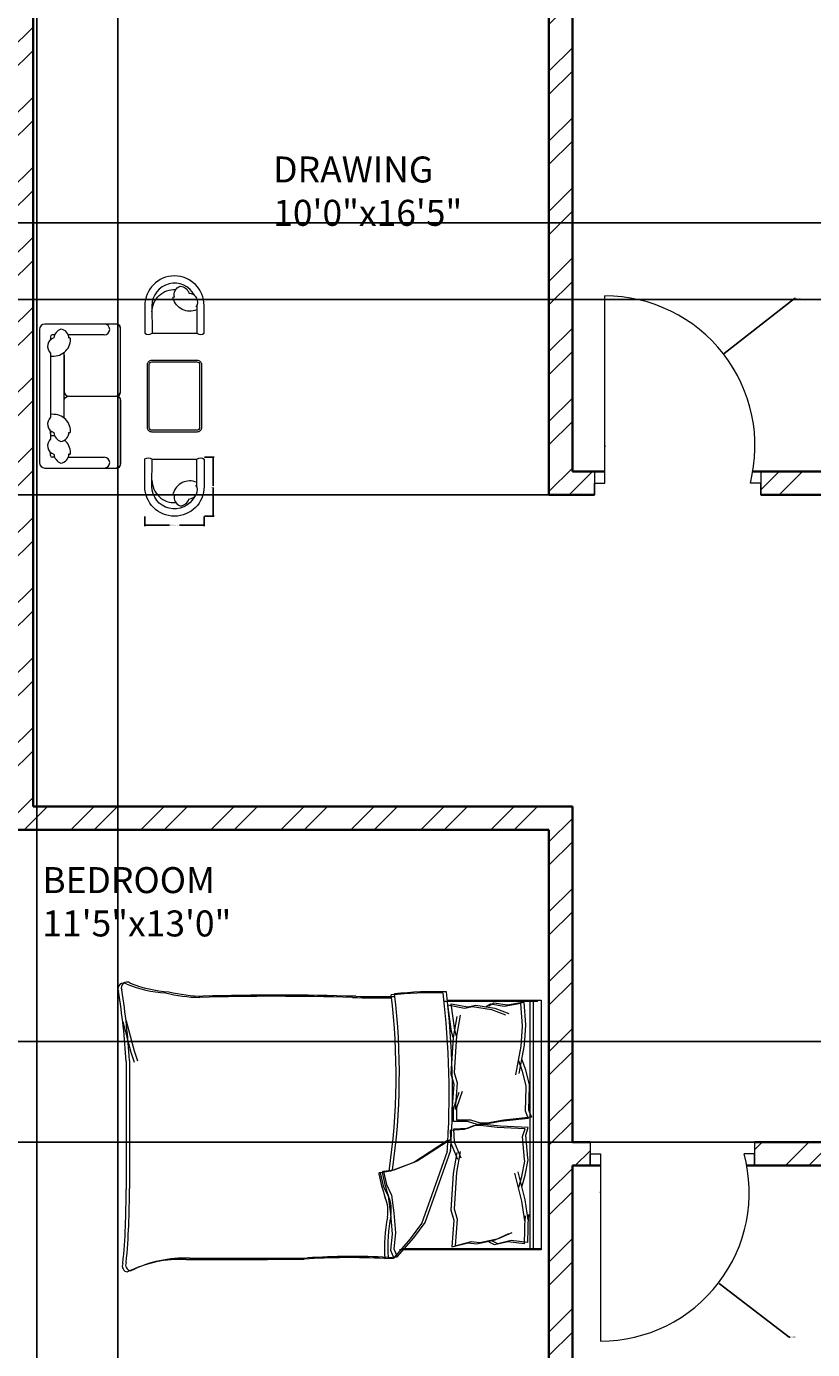
# Model space of a CAD drawing. Units: inches. Extents: x 2008 to 2657, y 1077 to 2165.
# Tile 6 of 16: x 2306 to 2457, y 1312 to 1567. Entities that reach past the tile are written whole.
import ezdxf

# ---------------------------------------------------------------- set-up
doc = ezdxf.new("R2010")
doc.units = ezdxf.units.IN
for name, color, linetype, lineweight in [('A-ANNO-DIMS', 2, 'Continuous', 18), ('A-AREA-IDEN', 4, 'Continuous', 18), ('A-DOOR', 11, 'Continuous', 18), ('A-FURN', 8, 'Continuous', 13), ('A-WALL', 7, 'Continuous', 35)]:
    doc.layers.add(name, color=color, linetype=linetype, lineweight=lineweight)
doc.layers.add('A-WALL-PATT', color=30, linetype='Continuous', lineweight=13, true_color=0xf8991e)
doc.styles.get("Standard").update_dxf_attribs({"font": 'arial.ttf'})
doc.dimstyles.get("Standard").update_dxf_attribs({"dimtxt": 0.18, "dimasz": 0.18, "dimexe": 0.18, "dimexo": 0.0625, "dimgap": 0.09, "dimtad": 0, "dimtih": 1, "dimtoh": 1, "dimdec": 4, "dimzin": 0, "dimdsep": 46, "dimtxsty": 'Standard', "dimcen": 0.09, "dimadec": 0, "dimazin": 0, "dimtfac": 1, "dimtdec": 4, "dimtofl": 0, "dimtmove": 0, "dimatfit": 3, "dimfxl": 1, "dimtolj": 1, "dimtzin": 0, "dimarcsym": 0})

# ---------------------------------------------------------------- blocks, each defined once
blk = doc.blocks.new('A$C1352')
at = {"color": 0}
for points in [[(0.003, 0.053), (0.003, 0.553, -0.414214), (0.053, 0.603), (0.753, 0.603, -0.414214), (0.803, 0.553), (0.803, 0.053, -0.414214), (0.753, 0.003), (0.053, 0.003, -0.414214)], [(0.023, 0.053), (0.023, 0.553, -0.414214), (0.053, 0.583), (0.753, 0.583, -0.414214), (0.783, 0.553), (0.783, 0.053, -0.414214), (0.753, 0.023), (0.053, 0.023, -0.414214)]]:
    blk.add_lwpolyline(points, format="xyb", close=True, dxfattribs=at)
blk = doc.blocks.new('BED-DOUBLE')
for p, q in [((0, 51.49), (0.64, 51.49)), ((0, 3.48), (0, 51.49)), ((0, 51.27), (26.61, 51.27)), ((0, 51.27), (26.61, 51.27)), ((0.64, 51.49), (27.25, 51.49)), ((0.64, 51.49), (27.25, 51.49)), ((1.53, 3.48), (1.53, 51.27)), ((1.53, 3.48), (1.53, 51.27)), ((2.17, 3.7), (2.17, 51.49)), ((2.17, 3.7), (2.17, 51.49)), ((17.21, 50.93), (14.07, 50.15)), ((17.21, 50.93), (14.07, 50.15)), ((16.81, 45.8), (17.21, 50.93)), ((16.81, 45.8), (17.21, 50.93)), ((27.75, 52.87), (24.5, 49.16)), ((27.75, 52.87), (24.5, 49.16)), ((28.39, 53.1), (25.14, 49.39)), ((28.39, 53.1), (25.14, 49.39)), ((29.49, 52.95), (27.75, 52.87, 3.87)), ((29.49, 52.95), (27.75, 52.87, 3.87)), ((28.37, 51.33), (27.75, 52.87)), ((28.37, 51.33), (27.75, 52.87)), ((28.06, 48.23), (28.37, 51.33)), ((28.06, 48.23), (28.37, 51.33)), ((30.13, 53.18), (28.39, 53.1, 3.87)), ((30.13, 53.18), (28.39, 53.1, 3.87)), ((29, 51.56), (28.39, 53.1)), ((29, 51.56), (28.39, 53.1)), ((28.7, 48.46), (29, 51.56)), ((28.7, 48.46), (29, 51.56)), ((2.56, 50.11), (2.46, 44.71)), ((2.56, 50.11), (2.46, 44.71)), ((2.56, 50.11), (5.77, 49.73)), ((2.56, 50.11), (5.77, 49.73)), ((3.2, 50.34), (3.1, 44.94)), ((3.2, 50.34), (3.1, 44.94)), ((3.2, 50.34), (6.41, 49.96)), ((3.2, 50.34), (6.41, 49.96)), ((8.26, 49.31), (5.58, 48.13)), ((8.26, 49.31), (5.58, 48.13)), ((5.77, 49.73), (8.34, 50.33)), ((5.77, 49.73), (8.34, 50.33)), ((8.9, 49.54), (6.22, 48.36)), ((8.9, 49.54), (6.22, 48.36)), ((6.41, 49.96), (8.98, 50.56)), ((6.41, 49.96), (8.98, 50.56)), ((11.83, 50.11), (8.26, 49.31)), ((11.83, 50.11), (8.26, 49.31)), ((8.34, 50.33), (9.38, 49.82)), ((8.34, 50.33), (9.38, 49.81)), ((12.47, 50.34), (8.9, 49.54)), ((12.47, 50.34), (8.9, 49.54)), ((8.98, 50.56), (10.02, 50.04)), ((8.98, 50.56), (10.02, 50.04)), ((13.43, 49.92), (11.83, 50.11)), ((13.43, 49.92), (11.83, 50.11)), ((14.07, 50.15), (12.47, 50.34)), ((14.07, 50.15), (12.47, 50.34)), ((16.57, 50.7), (13.43, 49.92)), ((16.57, 50.7), (13.43, 49.92)), ((16.17, 45.57), (16.57, 50.7)), ((16.17, 45.57), (16.57, 50.7)), ((24.5, 49.16), (22.33, 46.22)), ((24.5, 49.16), (22.33, 46.22)), ((25.14, 49.39), (22.97, 46.45)), ((25.14, 49.39), (22.97, 46.45)), ((29, 44.59), (28.7, 48.46)), ((29, 44.59), (28.7, 48.46)), ((3.1, 44.94), (3.18, 45.94)), ((3.1, 44.94), (3.18, 45.94)), ((3.18, 45.94), (3.71, 42.14)), ((3.18, 45.94), (3.71, 42.14)), ((22.33, 46.22), (20.32, 40.64)), ((22.33, 46.22), (20.32, 40.64)), ((22.97, 46.45), (20.96, 40.87)), ((22.97, 46.45), (20.96, 40.87)), ((28.37, 44.36), (28.06, 48.23)), ((28.37, 44.36), (28.06, 48.23)), ((2.46, 44.71), (2.54, 45.71)), ((2.46, 44.71), (2.54, 45.71)), ((2.54, 45.71), (3.07, 41.91)), ((2.54, 45.71), (3.07, 41.91)), ((16.73, 43.61), (16.17, 45.57)), ((16.73, 43.61), (16.17, 45.57)), ((16.3, 36.6), (16.73, 43.61)), ((16.3, 36.6), (16.73, 43.61)), ((17.37, 43.84), (16.81, 45.8)), ((17.37, 43.83), (16.81, 45.8)), ((16.93, 36.83), (17.37, 43.84)), ((16.93, 36.82), (17.37, 43.83)), ((28.83, 40.95), (28.37, 44.36)), ((28.83, 40.95), (28.37, 44.36)), ((29.47, 41.18), (29, 44.59)), ((29.47, 41.18), (29, 44.59)), ((3.07, 41.91), (4.42, 36.5)), ((3.07, 41.91), (4.42, 36.5)), ((3.71, 42.14), (5.06, 36.72)), ((3.71, 42.14), (5.06, 36.72)), ((20.96, 40.87), (18.02, 32.54)), ((20.96, 40.87), (18.02, 32.53)), ((29.76, 38.94), (28.83, 40.95)), ((29.76, 38.94), (28.83, 40.95)), ((30.4, 39.17), (29.47, 41.18)), ((30.4, 39.17), (29.47, 41.18)), ((3.67, 39.2), (3.08, 37.14)), ((3.67, 39.2), (3.08, 37.14)), ((4.31, 39.43), (3.72, 37.36)), ((4.31, 39.43), (3.72, 37.36)), ((20.32, 40.64), (17.38, 32.31)), ((20.32, 40.64), (17.38, 32.31)), ((30.38, 36.46), (29.76, 38.94)), ((30.38, 36.46), (29.76, 38.94)), ((31.02, 36.69), (30.4, 39.17)), ((31.02, 36.69), (30.4, 39.17)), ((79.25, 15.06), (79.25, 39.68)), ((79.25, 15.06), (79.25, 39.68)), ((79.88, 15.29), (79.88, 39.91)), ((79.88, 15.29), (79.88, 39.91)), ((3.08, 37.14), (2.54, 34.21)), ((3.08, 37.14), (2.54, 34.2)), ((3.72, 37.36), (3.18, 34.43)), ((3.72, 37.36), (3.18, 34.43)), ((15.63, 32.56), (16.3, 36.6)), ((15.63, 32.56), (16.3, 36.6)), ((16.27, 32.79), (16.93, 36.83)), ((16.27, 32.79), (16.93, 36.82)), ((23.88, 34.45), (28.37, 36.15)), ((23.88, 34.45), (28.37, 36.15)), ((24.52, 34.68), (29, 36.38)), ((24.52, 34.68), (29, 36.38)), ((28.37, 36.15), (30.38, 36.46)), ((28.37, 36.15), (30.38, 36.46)), ((29, 36.38), (31.02, 36.69)), ((29, 36.38), (31.02, 36.69)), ((2.54, 34.21), (2.56, 33.88)), ((2.54, 34.2), (2.56, 33.88)), ((2.56, 33.88), (2.98, 29.46)), ((2.56, 33.88), (2.98, 29.46)), ((3.18, 34.43), (3.2, 34.11)), ((3.18, 34.43), (3.2, 34.11)), ((3.2, 34.11), (3.62, 29.68)), ((3.2, 34.11), (3.62, 29.68)), ((16.74, 30.75), (15.45, 33.82)), ((16.74, 30.75), (15.45, 33.82)), ((17.38, 30.98), (16.09, 34.05)), ((17.38, 30.98), (16.09, 34.05)), ((17.38, 30.26), (23.88, 34.45)), ((17.38, 30.26), (23.88, 34.45)), ((18.02, 30.49), (24.52, 34.68)), ((18.02, 30.49), (24.52, 34.68)), ((16.89, 28.3), (16.74, 30.75)), ((16.89, 28.3), (16.74, 30.75)), ((17.53, 28.53), (17.38, 30.98)), ((17.53, 28.53), (17.38, 30.98)), ((2.98, 29.46), (2.49, 27.98)), ((2.98, 29.46), (2.49, 27.98)), ((3.62, 29.68), (3.13, 28.21)), ((3.62, 29.68), (3.13, 28.21)), ((3.13, 28.21), (8.51, 27.96)), ((3.13, 28.21), (8.51, 27.96)), ((12.38, 27.44), (14.22, 28.13)), ((12.38, 27.44), (14.22, 28.13)), ((13.02, 27.66), (14.86, 28.36)), ((13.02, 27.66), (14.86, 28.36)), ((14.22, 28.13), (16.89, 28.3)), ((14.22, 28.13), (16.89, 28.3)), ((14.86, 28.36), (17.53, 28.53)), ((14.86, 28.36), (17.53, 28.53)), ((1.87, 25.98), (7.22, 26.56)), ((1.87, 25.98), (7.22, 26.56)), ((2.45, 24.54), (1.87, 25.98)), ((2.45, 24.54), (1.87, 25.98)), ((2.49, 27.98), (7.87, 27.73)), ((2.49, 27.98), (7.87, 27.73)), ((2.51, 26.21), (7.86, 26.79)), ((2.51, 26.21), (7.86, 26.79)), ((3.09, 24.77), (2.51, 26.21)), ((3.09, 24.77), (2.51, 26.21)), ((7.22, 26.56), (10.4, 27.14)), ((7.22, 26.56), (10.4, 27.14)), ((7.86, 26.79), (11.04, 27.37)), ((7.86, 26.79), (11.04, 27.37)), ((7.87, 27.73), (11.08, 27.36)), ((7.87, 27.73), (11.08, 27.36)), ((8.51, 27.96), (11.72, 27.58)), ((8.51, 27.96), (11.72, 27.58)), ((10.4, 27.14), (11.7, 27.14)), ((10.4, 27.14), (11.7, 27.14)), ((11.04, 27.37), (12.34, 27.37)), ((11.04, 27.37), (12.34, 27.37)), ((11.08, 27.36), (12.38, 27.44)), ((11.08, 27.36), (12.38, 27.44)), ((11.7, 27.14), (13.58, 26.56)), ((11.7, 27.14), (13.58, 26.56)), ((11.72, 27.58), (13.02, 27.66)), ((11.72, 27.58), (13.02, 27.66)), ((12.34, 27.37), (14.22, 26.79)), ((12.34, 27.37), (14.22, 26.79)), ((13.58, 26.56), (16.26, 26.56)), ((13.58, 26.56), (16.26, 26.56)), ((14.22, 26.79), (16.9, 26.79)), ((14.22, 26.79), (16.9, 26.79)), ((16.26, 26.56), (16.26, 24.1)), ((16.26, 26.56), (16.26, 24.1)), ((16.9, 26.79), (16.9, 24.33)), ((16.9, 26.79), (16.9, 24.33)), ((2.3, 20.09), (2.45, 24.54)), ((2.3, 20.09), (2.45, 24.54)), ((2.94, 20.32), (3.09, 24.77)), ((2.94, 20.32), (3.09, 24.77)), ((16.26, 24.1), (15.17, 20.96)), ((16.26, 24.1), (15.17, 20.96)), ((16.9, 24.33), (15.81, 21.19)), ((16.9, 24.33), (15.81, 21.19)), ((16.17, 19.38), (16.57, 24.52)), ((16.17, 19.38), (16.57, 24.52)), ((16.81, 19.61), (17.21, 24.74)), ((16.81, 19.61), (17.21, 24.74)), ((2.3, 19.77), (2.3, 20.09)), ((2.3, 19.77), (2.3, 20.09)), ((3.03, 16.88), (2.3, 19.77)), ((3.03, 16.88), (2.3, 19.77)), ((2.94, 20), (2.94, 20.32)), ((2.94, 20), (2.94, 20.32)), ((3.67, 17.11), (2.94, 20)), ((3.67, 17.11), (2.94, 20)), ((3.96, 12.34), (4.97, 17.83)), ((3.96, 12.34), (4.97, 17.83)), ((16.73, 17.42), (16.17, 19.38)), ((16.73, 17.42), (16.17, 19.38)), ((17.37, 17.65), (16.81, 19.61)), ((17.37, 17.65), (16.81, 19.61)), ((3.75, 14.86), (3.03, 16.88)), ((3.75, 14.86), (3.03, 16.88)), ((3.32, 12.11), (4.33, 17.6)), ((3.32, 12.11), (4.33, 17.6)), ((4.39, 15.08), (3.67, 17.11)), ((4.39, 15.08), (3.67, 17.11)), ((16.3, 10.41), (16.73, 17.42)), ((16.3, 10.41), (16.73, 17.42)), ((16.93, 10.64), (17.37, 17.65)), ((16.93, 10.64), (17.37, 17.65)), ((3.03, 8.29), (3.32, 12.11)), ((3.03, 8.29), (3.32, 12.11)), ((3.67, 8.51), (3.96, 12.34)), ((3.67, 8.51), (3.96, 12.34)), ((15.63, 6.38), (16.3, 10.41)), ((15.63, 6.38), (16.3, 10.41)), ((16.27, 6.61), (16.93, 10.64)), ((16.27, 6.61), (16.93, 10.64)), ((16.3, 10.41), (16.62, 9.28)), ((16.3, 10.41), (16.62, 9.28)), ((16.93, 10.64), (17.26, 9.51)), ((16.93, 10.64), (17.26, 9.51)), ((3.01, 8.18), (3.03, 8.29)), ((3.01, 8.18), (3.03, 8.29)), ((3.34, 3.9), (3.01, 8.18)), ((3.34, 3.9), (3.01, 8.18)), ((3.65, 8.41), (3.67, 8.51)), ((3.65, 8.41), (3.67, 8.51)), ((3.98, 4.13), (3.65, 8.41)), ((3.98, 4.13), (3.65, 8.41)), ((16.62, 9.28), (17.34, 4.18)), ((16.62, 9.28), (17.34, 4.18)), ((17.26, 9.51), (17.98, 4.41)), ((17.26, 9.51), (17.98, 4.41)), ((8.96, 5.05), (6.21, 6.06)), ((8.96, 5.05), (6.21, 6.06)), ((9.59, 5.28), (6.85, 6.29)), ((9.59, 5.28), (6.85, 6.29)), ((13.21, 4.7), (9.59, 5.28)), ((13.21, 4.7), (9.59, 5.28)), ((18.11, 3.48), (0, 3.48)), ((18.11, 3.48), (0, 3.48)), ((18.75, 3.7), (0.64, 3.7)), ((18.75, 3.7), (0.64, 3.7)), ((3.32, 3.9), (6.5, 4.47)), ((3.32, 3.89), (6.5, 4.47)), ((3.96, 4.12), (7.14, 4.7)), ((3.96, 4.12), (7.14, 4.7)), ((6.5, 4.47), (9.1, 4.04)), ((6.5, 4.47), (9.1, 4.04)), ((7.14, 4.7), (9.74, 4.27)), ((7.14, 4.7), (9.74, 4.27)), ((12.57, 4.47), (8.96, 5.05)), ((12.57, 4.47), (8.96, 5.05)), ((9.1, 4.04), (10.11, 4.62)), ((9.1, 4.04), (10.11, 4.62)), ((9.74, 4.27), (10.75, 4.85)), ((9.74, 4.27), (10.75, 4.85)), ((14.16, 4.76), (12.57, 4.47)), ((14.16, 4.76), (12.57, 4.47)), ((14.8, 4.99), (13.21, 4.7)), ((14.8, 4.99), (13.21, 4.7)), ((17.34, 4.18), (14.16, 4.76)), ((17.34, 4.18), (14.16, 4.76)), ((17.98, 4.41), (14.8, 4.99)), ((17.98, 4.41), (14.8, 4.99))]:
    blk.add_line(p, q)
for centre, radius, start, end in [((68.67, 76.16), 23.07, 267.4714, 296.4681), ((68.67, 76.16), 23.07, 267.4714, 296.4681), ((69.31, 76.39), 23.07, 267.4714, 296.4681), ((69.31, 76.39), 23.07, 267.4714, 296.4681), ((78.87, 54.41), 1.1, 332.6588, 86.02), ((78.87, 54.41), 1.1, 332.6588, 86.02), ((212.28, 41.15), 133.04, 174.4998, 180.6351), ((212.28, 41.15), 133.04, 174.4998, 180.6351), ((79.51, 54.64), 1.1, 332.6588, 86.02), ((79.51, 54.64), 1.1, 332.6588, 86.02), ((212.92, 41.38), 133.04, 174.4998, 180.6351), ((212.92, 41.38), 133.04, 174.4998, 180.6351), ((-6.66, 51.33), 36.18, 349.8763, 2.5657), ((-6.66, 51.33), 36.18, 349.8763, 2.5657), ((36.32, 182.27), 129.5, 266.9791, 273.8365), ((36.32, 182.27), 129.5, 266.9791, 273.8365), ((-6.02, 51.56), 36.18, 349.8763, 2.5657), ((-6.02, 51.56), 36.18, 349.8763, 2.5657), ((36.95, 182.49), 129.5, 266.9791, 273.8365), ((36.95, 182.49), 129.5, 266.9791, 273.8365), ((67.82, -4508.74), 4561.86, 90.00217, 90.28689), ((67.82, -4508.74), 4561.86, 90.00217, 90.28689), ((68.46, -4508.51), 4561.86, 90.00217, 90.28689), ((68.46, -4508.51), 4561.86, 90.00217, 90.28689), ((35.07, 43.74), 6.22, 168.6608, 203.7384), ((35.07, 43.74), 6.22, 168.6608, 203.7384), ((35.71, 43.97), 6.22, 168.6608, 203.7384), ((35.71, 43.97), 6.22, 168.6608, 203.7384), ((1.48, 31.15), 29.65, 10.6617, 19.8806), ((1.48, 31.15), 29.65, 10.6617, 19.8806), ((2.12, 31.38), 29.65, 10.6617, 19.8806), ((2.12, 31.38), 29.65, 10.6617, 19.8806), ((156.32, 17.76), 129.02, 171.7845, 186.9006), ((156.32, 17.76), 129.02, 171.7845, 186.9006), ((156.96, 17.98), 129.02, 171.7845, 186.9006), ((156.96, 17.98), 129.02, 171.7845, 186.9006), ((30.44, 36.64), 0.185, 250.2464, 1.1377), ((30.44, 36.64), 0.185, 250.2464, 1.1377), ((31.08, 36.87), 0.185, 250.2464, 1.1377), ((31.08, 36.86), 0.185, 250.2464, 1.1377), ((182.05, 21.36), 164.97, 176.0865, 186.7821), ((182.05, 21.36), 164.97, 176.0865, 186.7821), ((182.69, 21.59), 164.97, 176.0865, 186.7821), ((182.69, 21.59), 164.97, 176.0865, 186.7821), ((-23.07, -16.99), 106.46, 13.3832, 17.7053), ((-23.07, -16.99), 106.46, 13.3832, 17.7053), ((201.48, 21.66), 121.76, 182.9958, 189.4091), ((201.48, 21.66), 121.76, 182.9958, 189.4091), ((-23.71, -17.22), 106.46, 13.3832, 17.7053), ((-23.71, -17.22), 106.46, 13.3832, 17.7053), ((200.84, 21.43), 121.76, 182.9958, 189.4091), ((200.84, 21.43), 121.76, 182.9958, 189.4091), ((31.17, -167.31), 170.11, 88.4762, 91.0082), ((31.17, -167.31), 170.11, 88.4762, 91.0082), ((31.81, -167.08), 170.11, 88.4762, 91.0082), ((31.81, -167.08), 170.11, 88.4762, 91.0082), ((50.61, 484.82), 482.31, 268.2277, 271.7185), ((50.61, 484.82), 482.31, 268.2277, 271.7185), ((51.25, 485.05), 482.31, 268.2277, 271.7185), ((51.25, 485.05), 482.31, 268.2277, 271.7185), ((64.52, -26.9), 29.63, 76.0648, 88.9113), ((64.52, -26.9), 29.63, 76.0648, 88.9113), ((65.15, -26.67), 29.63, 76.0648, 88.9113), ((65.15, -26.67), 29.63, 76.0648, 88.9113), ((20.1, 85.16), 83.31, 268.7218, 275.604), ((20.1, 85.16), 83.31, 268.7218, 275.604), ((20.74, 85.39), 83.31, 268.7218, 275.604), ((20.74, 85.39), 83.31, 268.7218, 275.604), ((70.28, -21.66), 23.56, 67.9751, 86.652), ((70.28, -21.66), 23.56, 67.9751, 86.652), ((70.92, -21.43), 23.56, 67.9751, 86.652), ((70.92, -21.43), 23.56, 67.9751, 86.652), ((79.72, 1.09), 1.09, 236.1736, 23.4781), ((79.72, 1.09), 1.09, 236.1736, 23.4781), ((80.36, 1.32), 1.09, 236.1736, 23.4781), ((80.36, 1.32), 1.09, 236.1736, 23.4781)]:
    blk.add_arc(centre, radius, start, end)
blk = doc.blocks.new('LOUNGE-CHAIR')
blk.add_line((1.39, 5.54), (1.38, 0.26))
at = {"ltscale": 0.03}
blk.add_lwpolyline([(1.38, 0.26, -0.369229), (0, 0.27), (0, 5.54, -1), (11.42, 5.53), (11.42, 0.25, -0.369229), (10.03, 0.26)], format="xyb", close=True, dxfattribs=at)
blk.add_lwpolyline([(1.88, 7.54, -0.785087), (10.04, 5.53), (10.03, 0.26)], format="xyb")
for centre, radius, start, end in [((3.01, 6.23), 1.73, 92.9922, 214.1401), ((4.77, 7.34), 1.95, 94.9999, 161.3534), ((3.98, 7.61), 1.78, 346.6403, 69.4695), ((5.71, 4.32), 4.33, 359.9461, 93.658), ((5.71, 5.54), 4.33, 178.8536, 179.9461), ((2.75, 7.82), 3.35, 247.0143, 344.2857), ((5.79, 7.01), 0.207, 330.6238, 113.7423)]:
    blk.add_arc(centre, radius, start, end)
blk = doc.blocks.new('*D15')
at = {"layer": 'A-ANNO-DIMS', "color": 0, "lineweight": -2, "transparency": 16777216}
for p, q in [((2329, 1472.5), (2329, 1470.67)), ((2329.18, 1470.85), (2333.76, 1470.85)), ((2340.24, 1470.85), (2335.66, 1470.85)), ((2340.42, 1472.5), (2340.42, 1470.67))]:
    blk.add_line(p, q, dxfattribs=at)
at = {"layer": 'A-ANNO-DIMS', "color": 0, "transparency": 16777216}
for points in [[(2329.18, 1470.88), (2329.18, 1470.82), (2329, 1470.85)], [(2340.24, 1470.88), (2340.24, 1470.82), (2340.42, 1470.85)]]:
    blk.add_solid(points, dxfattribs=at)
at = {"layer": 'Defpoints', "color": 0, "transparency": 16777216}
for p in [(2329, 1472.56), (2329, 1470.85), (2340.42, 1472.56)]:
    blk.add_point(p, dxfattribs=at)
at = {"layer": 'A-ANNO-DIMS', "color": 0, "transparency": 16777216, "insert": (2334.71, 1470.85), "char_height": 0.18, "attachment_point": 5}
blk.add_mtext('\\A1;CHAIR 11 TYP.', dxfattribs=at)
blk = doc.blocks.new('*D16')
at = {"layer": 'A-ANNO-DIMS', "color": 0, "lineweight": -2, "transparency": 16777216}
for p, q in [((2340.49, 1483.9), (2342.32, 1483.9)), ((2342.14, 1483.72), (2342.14, 1478.41)), ((2342.14, 1472.74), (2342.14, 1478.05)), ((2340.49, 1472.56), (2342.32, 1472.56))]:
    blk.add_line(p, q, dxfattribs=at)
at = {"layer": 'A-ANNO-DIMS', "color": 0, "transparency": 16777216}
for points in [[(2342.11, 1483.72), (2342.17, 1483.72), (2342.14, 1483.9)], [(2342.11, 1472.74), (2342.17, 1472.74), (2342.14, 1472.56)]]:
    blk.add_solid(points, dxfattribs=at)
at = {"layer": 'Defpoints', "color": 0, "transparency": 16777216}
for p in [(2340.42, 1483.9), (2340.42, 1472.56), (2342.14, 1472.56)]:
    blk.add_point(p, dxfattribs=at)
at = {"layer": 'A-ANNO-DIMS', "color": 0, "transparency": 16777216, "insert": (2342.14, 1478.23), "char_height": 0.18, "attachment_point": 5}
blk.add_mtext('\\A1;11 TYP.', dxfattribs=at)
blk = doc.blocks.new('*D31')
at = {"layer": 'A-ANNO-DIMS', "color": 0, "lineweight": -2, "transparency": 16777216}
for p, q in [((2076.26, 1562.18), (2076.26, 1140.44)), ((2576.76, 1188.61), (2576.76, 1140.44)), ((2076.44, 1140.62), (2326.12, 1140.62)), ((2576.58, 1140.62), (2326.91, 1140.62))]:
    blk.add_line(p, q, dxfattribs=at)
at = {"layer": 'A-ANNO-DIMS', "color": 0, "transparency": 16777216}
for points in [[(2076.44, 1140.65), (2076.44, 1140.59), (2076.26, 1140.62)], [(2576.58, 1140.65), (2576.58, 1140.59), (2576.76, 1140.62)]]:
    blk.add_solid(points, dxfattribs=at)
at = {"layer": 'Defpoints', "color": 0, "transparency": 16777216}
for p in [(2076.26, 1562.24), (2576.76, 1188.67), (2576.76, 1140.62)]:
    blk.add_point(p, dxfattribs=at)
at = {"layer": 'A-ANNO-DIMS', "color": 0, "transparency": 16777216, "insert": (2326.51, 1140.62), "char_height": 0.18, "attachment_point": 5}
blk.add_mtext('\\A1;500.5', dxfattribs=at)
blk = doc.blocks.new('*D53')
at = {"layer": 'A-ANNO-DIMS', "color": 0, "lineweight": -2, "transparency": 16777216}
for p, q in [((2406.7, 1613.17), (2028.03, 1613.17)), ((2028.21, 1612.99), (2028.21, 1545.11)), ((2028.21, 1476.85), (2028.21, 1544.74)), ((2406.7, 1476.67), (2028.03, 1476.67))]:
    blk.add_line(p, q, dxfattribs=at)
at = {"layer": 'A-ANNO-DIMS', "color": 0, "transparency": 16777216}
for points in [[(2028.18, 1612.99), (2028.24, 1612.99), (2028.21, 1613.17)], [(2028.18, 1476.85), (2028.24, 1476.85), (2028.21, 1476.67)]]:
    blk.add_solid(points, dxfattribs=at)
at = {"layer": 'Defpoints', "color": 0, "transparency": 16777216}
for p in [(2406.76, 1613.17), (2028.21, 1476.67), (2406.76, 1476.67)]:
    blk.add_point(p, dxfattribs=at)
at = {"layer": 'A-ANNO-DIMS', "color": 0, "transparency": 16777216, "insert": (2028.21, 1544.92), "char_height": 0.18, "attachment_point": 5}
blk.add_mtext('\\A1;136.5', dxfattribs=at)
blk = doc.blocks.new('*D64')
at = {"layer": 'A-ANNO-DIMS', "color": 0, "lineweight": -2, "transparency": 16777216}
for p, q in [((2308.25, 1777.08), (2308.25, 1140.44)), ((2323.83, 1776.91), (2323.83, 1140.44)), ((2308.43, 1140.62), (2315.59, 1140.62)), ((2323.65, 1140.62), (2316.49, 1140.62))]:
    blk.add_line(p, q, dxfattribs=at)
at = {"layer": 'A-ANNO-DIMS', "color": 0, "transparency": 16777216}
for points in [[(2308.43, 1140.65), (2308.43, 1140.59), (2308.25, 1140.62)], [(2323.65, 1140.65), (2323.65, 1140.59), (2323.83, 1140.62)]]:
    blk.add_solid(points, dxfattribs=at)
at = {"layer": 'Defpoints', "color": 0, "transparency": 16777216}
for p in [(2308.25, 1777.15), (2323.83, 1776.97), (2323.83, 1140.62)]:
    blk.add_point(p, dxfattribs=at)
at = {"layer": 'A-ANNO-DIMS', "color": 0, "transparency": 16777216, "insert": (2316.04, 1140.62), "char_height": 0.18, "attachment_point": 5}
blk.add_mtext('\\A1;15.572', dxfattribs=at)
blk = doc.blocks.new('*D68')
at = {"layer": 'A-ANNO-DIMS', "color": 0, "lineweight": -2, "transparency": 16777216}
for p, q in [((2572.2, 1371.57), (2028.03, 1371.57)), ((2028.21, 1371.39), (2028.21, 1362.05)), ((2028.21, 1352.35), (2028.21, 1361.69)), ((2572.2, 1352.17), (2028.03, 1352.17))]:
    blk.add_line(p, q, dxfattribs=at)
at = {"layer": 'A-ANNO-DIMS', "color": 0, "transparency": 16777216}
for points in [[(2028.18, 1371.39), (2028.24, 1371.39), (2028.21, 1371.57)], [(2028.18, 1352.35), (2028.24, 1352.35), (2028.21, 1352.17)]]:
    blk.add_solid(points, dxfattribs=at)
at = {"layer": 'Defpoints', "color": 0, "transparency": 16777216}
for p in [(2028.21, 1371.57), (2572.26, 1371.57), (2572.26, 1352.17)]:
    blk.add_point(p, dxfattribs=at)
at = {"layer": 'A-ANNO-DIMS', "color": 0, "transparency": 16777216, "insert": (2028.21, 1361.87), "char_height": 0.18, "attachment_point": 5}
blk.add_mtext('\\A1;19.394', dxfattribs=at)
blk = doc.blocks.new('*D69')
at = {"layer": 'A-ANNO-DIMS', "color": 0, "lineweight": -2, "transparency": 16777216}
for p, q in [((2109.32, 1529), (2624.99, 1529)), ((2624.81, 1528.82), (2624.81, 1521.8)), ((2624.81, 1514.42), (2624.81, 1521.44)), ((2109.32, 1514.24), (2624.99, 1514.24))]:
    blk.add_line(p, q, dxfattribs=at)
at = {"layer": 'A-ANNO-DIMS', "color": 0, "transparency": 16777216}
for points in [[(2624.78, 1528.82), (2624.84, 1528.82), (2624.81, 1529)], [(2624.78, 1514.42), (2624.84, 1514.42), (2624.81, 1514.24)]]:
    blk.add_solid(points, dxfattribs=at)
at = {"layer": 'Defpoints', "color": 0, "transparency": 16777216}
for p in [(2109.26, 1529), (2624.81, 1529), (2109.26, 1514.24)]:
    blk.add_point(p, dxfattribs=at)
at = {"layer": 'A-ANNO-DIMS', "color": 0, "transparency": 16777216, "insert": (2624.81, 1521.62), "char_height": 0.18, "attachment_point": 5}
blk.add_mtext('\\A1;14.756', dxfattribs=at)
blk = doc.blocks.new('*D71')
at = {"layer": 'A-ANNO-DIMS', "color": 0, "lineweight": -2, "transparency": 16777216}
for p, q in [((2454.01, 1514.4), (2440.47, 1503.88)), ((2454.19, 1514.4), (2454.01, 1514.4)), ((2417.44, 1486.05), (2417.62, 1486.05)), ((2417.53, 1485.96), (2417.53, 1486.14))]:
    blk.add_line(p, q, dxfattribs=at)
at = {"layer": 'A-ANNO-DIMS', "color": 0, "transparency": 16777216}
blk.add_solid([(2440.45, 1503.9), (2440.49, 1503.86), (2440.33, 1503.77)], dxfattribs=at)
at = {"layer": 'Defpoints', "color": 0, "transparency": 16777216}
for p in [(2440.33, 1503.77), (2417.53, 1486.05)]:
    blk.add_point(p, dxfattribs=at)
at = {"layer": 'A-ANNO-DIMS', "color": 0, "transparency": 16777216, "insert": (2454.74, 1514.4), "char_height": 0.18, "attachment_point": 5}
blk.add_mtext('\\A1;R28.873', dxfattribs=at)
blk = doc.blocks.new('*D73')
at = {"layer": 'A-ANNO-DIMS', "color": 0, "lineweight": -2, "transparency": 16777216}
for p, q in [((2416.61, 1342.52), (2416.79, 1342.52)), ((2416.7, 1342.43), (2416.7, 1342.61)), ((2453, 1314.67), (2439.53, 1325)), ((2453.18, 1314.67), (2453, 1314.67))]:
    blk.add_line(p, q, dxfattribs=at)
at = {"layer": 'A-ANNO-DIMS', "color": 0, "transparency": 16777216}
blk.add_solid([(2439.55, 1325.03), (2439.51, 1324.98), (2439.39, 1325.11)], dxfattribs=at)
at = {"layer": 'Defpoints', "color": 0, "transparency": 16777216}
for p in [(2416.7, 1342.52), (2439.39, 1325.11)]:
    blk.add_point(p, dxfattribs=at)
at = {"layer": 'A-ANNO-DIMS', "color": 0, "transparency": 16777216, "insert": (2453.73, 1314.67), "char_height": 0.18, "attachment_point": 5}
blk.add_mtext('\\A1;R28.593', dxfattribs=at)

msp = doc.modelspace()

# ---------------------------------------------------------------- hatches: boundary and pattern name
at = {"layer": 'A-WALL-PATT'}
h = msp.add_hatch(dxfattribs=at)
h.set_pattern_fill('ANSI32', color=256)
h.paths.add_polyline_path([(2109.2619, 2094.6743), (2104.7619, 2094.6743), (2104.7619, 2072.1743), (2104.7619, 2021.6151), (2109.2619, 2021.6151), (2109.2619, 2055.6743), (2126.1387, 2055.6743), (2126.1387, 2057.9243), (2126.1387, 2060.1743), (2109.2619, 2060.1743)])
h.paths.add_polyline_path([(2223.2494, 2057.9243), (2223.2494, 2060.1743), (2186.1387, 2060.1743), (2186.1387, 2055.6743), (2223.2494, 2055.6743)])
h.paths.add_polyline_path([(2250.7619, 2072.1743), (2250.7619, 2090.1743), (2250.7619, 2094.6743), (2246.2619, 2094.6743), (2246.2619, 2060.1743), (2242.7242, 2060.1743), (2242.7242, 2055.6743), (2246.2619, 2055.6743), (2246.2619, 1899.6743), (2242.7458, 1899.6743), (2242.7458, 1897.4243), (2242.7458, 1895.1743), (2246.2619, 1895.1743), (2246.2619, 1878.8745), (2248.5119, 1878.8745), (2250.7619, 1878.8745), (2250.7619, 1991.1743), (2250.7619, 2025.6743), (2257.6798, 2025.6743), (2257.6798, 2027.9243), (2257.6798, 2030.1743), (2250.7619, 2030.1743)])
h.paths.add_polyline_path([(2411.2619, 2031.6743), (2409.0119, 2031.6743), (2406.7619, 2031.6743), (2406.7619, 2030.1743), (2322.7619, 2030.1743), (2322.7619, 2053.3443), (2318.2619, 2053.3443), (2318.2619, 2030.1743), (2305.6798, 2030.1743), (2305.6798, 2025.6743), (2318.2619, 2025.6743), (2322.7619, 2025.6743), (2406.7619, 2025.6743), (2406.7619, 1995.6743), (2406.7619, 1847.2677), (2250.7619, 1847.2677), (2250.7619, 1850.9902), (2248.5119, 1850.9902), (2246.2619, 1850.9902), (2246.2619, 1847.1743), (2246.2619, 1842.7677), (2303.0015, 1842.7677), (2303.0015, 1667.2413), (2298.4208, 1667.2413), (2298.4208, 1662.7413), (2303.0015, 1662.7413), (2303.0015, 1649.8758), (2307.5015, 1649.8758), (2307.5015, 1842.7677), (2406.7619, 1842.7677), (2411.2619, 1842.7677), (2411.2619, 1878.6743), (2415.8196, 1878.6743), (2415.8196, 1880.9243), (2415.8196, 1883.1743), (2411.2619, 1883.1743)])
h.paths.add_polyline_path([(2411.2619, 2094.6743), (2406.7619, 2094.6743), (2318.2619, 2094.6743), (2318.2619, 2077.3443), (2322.7619, 2077.3443), (2322.7619, 2090.1743), (2406.7619, 2090.1743), (2406.7619, 2072.1743), (2406.7619, 2067.6743), (2406.7619, 2052.7524), (2411.2619, 2052.7524), (2411.2619, 2055.6743), (2414.9888, 2055.6743), (2414.9888, 2057.9243), (2414.9888, 2060.1743), (2411.2619, 2060.1743), (2411.2619, 2072.1743)])
h.paths.add_polyline_path([(2576.7619, 2072.1743), (2576.7619, 2094.6743), (2572.2619, 2094.6743), (2572.2619, 2060.1743), (2525.8113, 2060.1743), (2525.8113, 2055.6743), (2572.2619, 2055.6743), (2572.2619, 1994.289), (2576.7619, 1994.289)])
h.paths.add_polyline_path([(2465.8113, 2060.1743), (2436.2802, 2060.1743), (2436.2802, 2055.6743), (2465.8113, 2055.6743), (2465.8113, 2057.9243)])
h.paths.add_polyline_path([(2576.7619, 1934.289), (2574.5119, 1934.289), (2572.2619, 1934.289), (2572.2619, 1883.1743), (2447.7027, 1883.1743), (2447.7027, 1878.6743), (2459.7619, 1878.6743), (2459.7619, 1830.4982), (2464.2619, 1830.4982), (2464.2619, 1878.6743), (2572.2619, 1878.6743), (2572.2619, 1868.4883), (2576.7619, 1868.4883)])
h.paths.add_polyline_path([(2576.7619, 1832.4883), (2572.2619, 1832.4883), (2572.2619, 1806.6743), (2464.2619, 1806.6743), (2464.2619, 1809.6629), (2459.7619, 1809.6629), (2459.7619, 1802.1743), (2483.7619, 1802.1743), (2483.7619, 1778.1743), (2488.2619, 1778.1743), (2488.2619, 1802.1743), (2572.2619, 1802.1743), (2572.2619, 1793.6101), (2576.7619, 1793.6101)])
h.paths.add_polyline_path([(2576.7619, 1769.6101), (2572.2619, 1769.6101), (2572.2619, 1754.1743), (2488.2619, 1754.1743), (2488.2619, 1757.2675), (2486.0119, 1757.2675), (2483.7619, 1757.2675), (2483.7619, 1754.1743), (2447.4528, 1754.1743), (2447.4528, 1749.6743), (2483.7619, 1749.6743), (2572.2619, 1749.6743), (2572.2619, 1715.1837), (2576.7619, 1715.1837)])
h.paths.add_polyline_path([(2576.7619, 1655.1837), (2572.2619, 1655.1837), (2572.2619, 1617.6743), (2411.2619, 1617.6743), (2411.2619, 1749.6743), (2414.2827, 1749.6743), (2414.2827, 1754.1743), (2406.7619, 1754.1743), (2406.7619, 1749.6743), (2406.7619, 1617.6743), (2307.5015, 1617.6743), (2307.5015, 1621.0007), (2305.2515, 1621.0007), (2303.0015, 1621.0007), (2303.0015, 1609.6944), (2307.5015, 1609.6944), (2307.5015, 1613.1743), (2406.7619, 1613.1743), (2406.7619, 1476.6743), (2415.532, 1476.6743), (2415.532, 1478.9243), (2415.532, 1481.1743), (2411.2619, 1481.1743), (2411.2619, 1613.1743), (2572.2619, 1613.1743), (2572.2619, 1584.6086), (2576.7619, 1584.6086)])
h.paths.add_polyline_path([(2576.7619, 1524.6086), (2572.2619, 1524.6086), (2572.2619, 1481.1743), (2483.7619, 1481.1743), (2447.5119, 1481.1743), (2447.5119, 1476.6743), (2483.7619, 1476.6743), (2483.7619, 1473.5051), (2488.2619, 1473.5051), (2488.2619, 1476.6743), (2572.2619, 1476.6743), (2572.2619, 1469.5488), (2576.7619, 1469.5488)])
h.paths.add_polyline_path([(2576.7619, 1445.5488), (2572.2619, 1445.5488), (2572.2619, 1428.6743), (2488.2619, 1428.6743), (2488.2619, 1455.6743), (2486.0119, 1455.6743), (2483.7619, 1455.6743), (2483.7619, 1428.6743), (2459.7619, 1428.6743), (2459.7619, 1422.1519), (2464.2619, 1422.1519), (2464.2619, 1424.1743), (2572.2619, 1424.1743), (2572.2619, 1407.5685), (2576.7619, 1407.5685)])
h.paths.add_polyline_path([(2576.7619, 1371.5685), (2572.2619, 1371.5685), (2572.2619, 1352.1743), (2464.2619, 1352.1743), (2464.2619, 1403.1384), (2462.0119, 1403.1384), (2459.7619, 1403.1384), (2459.7619, 1352.1743), (2446.3194, 1352.1743), (2446.3194, 1347.6743), (2572.2619, 1347.6743), (2572.2619, 1321.0291), (2576.7619, 1321.0291)])
h.paths.add_polyline_path([(2462.703, 1227.6743), (2436.0298, 1227.6743), (2436.0298, 1225.4243), (2436.0298, 1223.1743), (2462.703, 1223.1743), (2462.703, 1225.4243)])
h.paths.add_polyline_path([(2576.7619, 1261.0291), (2574.5119, 1261.0291), (2572.2619, 1261.0291), (2572.2619, 1227.6743), (2522.703, 1227.6743), (2522.703, 1223.1743), (2572.2619, 1223.1743), (2572.2619, 1188.6743), (2576.7619, 1188.6743), (2576.7619, 1193.1743), (2576.7619, 1223.1743)])
h.paths.add_polyline_path([(2414.2823, 1227.6743), (2411.2619, 1227.6743), (2411.2619, 1267.1779), (2409.0119, 1267.1779), (2406.7619, 1267.1779), (2406.7619, 1227.6743), (2322.7619, 1227.6743), (2322.7619, 1244.3623), (2318.2619, 1244.3623), (2318.2619, 1223.1743), (2406.7619, 1223.1743), (2406.7619, 1193.1743), (2406.7619, 1188.6743), (2411.2619, 1188.6743), (2411.2619, 1193.1743), (2411.2619, 1223.1743), (2414.2823, 1223.1743)])
h.paths.add_polyline_path([(2411.2619, 1347.6743), (2414.702, 1347.6743), (2414.702, 1349.9243), (2414.702, 1352.1743), (2411.2619, 1352.1743), (2411.2619, 1416.7413), (2307.5015, 1416.7413), (2307.5015, 1579.8489), (2305.2515, 1579.8489), (2303.0015, 1579.8489), (2303.0015, 1566.7413), (2299.2719, 1566.7413), (2299.2719, 1562.2413), (2303.0015, 1562.2413), (2303.0015, 1416.7413), (2246.2619, 1416.7413), (2246.2619, 1409.8616), (2250.7619, 1409.8616), (2250.7619, 1412.2413), (2406.7619, 1412.2413), (2406.7619, 1292.1743), (2304.9703, 1292.1743), (2304.9703, 1287.6743), (2318.2619, 1287.6743), (2318.2619, 1268.3623), (2322.7619, 1268.3623), (2322.7619, 1287.6743), (2406.7619, 1287.6743), (2406.7619, 1285.4748), (2411.2619, 1285.4748)])
h.paths.add_polyline_path([(2109.2619, 1262.7482), (2104.7619, 1262.7482), (2104.7619, 1223.1743), (2104.7619, 1193.1743), (2104.7619, 1188.6743), (2109.2619, 1188.6743), (2109.2619, 1223.1743), (2126.7928, 1223.1743), (2126.7928, 1225.4243), (2126.7928, 1227.6743), (2109.2619, 1227.6743)])
h.paths.add_polyline_path([(2222.3268, 1227.6743), (2186.7928, 1227.6743), (2186.7928, 1223.1743), (2222.3268, 1223.1743)])
h.paths.add_polyline_path([(2250.7619, 1287.6743), (2256.9703, 1287.6743), (2256.9703, 1289.9243), (2256.9703, 1292.1743), (2250.7619, 1292.1743), (2250.7619, 1382.2078), (2248.5119, 1382.2078), (2246.2619, 1382.2078), (2246.2619, 1347.6743), (2246.2619, 1227.6743), (2242.6068, 1227.6743), (2242.6068, 1223.1743), (2246.2619, 1223.1743), (2246.2619, 1188.6743), (2250.7619, 1188.6743), (2250.7619, 1193.1743), (2250.7619, 1227.6743)])
h.paths.add_polyline_path([(2133.2619, 1349.9243), (2133.2619, 1352.1743), (2109.2619, 1352.1743), (2109.2619, 1375.2826), (2104.7619, 1375.2826), (2104.7619, 1322.7482), (2109.2619, 1322.7482), (2109.2619, 1347.6743), (2133.2619, 1347.6743)])
h.paths.add_polyline_path([(2210.2105, 1352.1743), (2161.7619, 1352.1743), (2161.7619, 1412.2413), (2185.7619, 1412.2413), (2185.7619, 1420.1851), (2183.5119, 1420.1851), (2181.2619, 1420.1851), (2181.2619, 1416.7413), (2109.2619, 1416.7413), (2109.2619, 1452.4006), (2104.7619, 1452.4006), (2104.7619, 1399.2826), (2109.2619, 1399.2826), (2109.2619, 1412.2413), (2157.2619, 1412.2413), (2157.2619, 1352.1743), (2154.3383, 1352.1743), (2154.3383, 1347.6743), (2210.2105, 1347.6743)])
h.paths.add_polyline_path([(2185.7619, 1514.2413), (2161.7619, 1514.2413), (2161.7619, 1518.1307), (2159.5119, 1518.1307), (2157.2619, 1518.1307), (2157.2619, 1514.2413), (2109.2619, 1514.2413), (2109.2619, 1528.997), (2107.0119, 1528.997), (2104.7619, 1528.997), (2104.7619, 1488.4006), (2109.2619, 1488.4006), (2109.2619, 1509.7413), (2181.2619, 1509.7413), (2181.2619, 1441.2042), (2185.7619, 1441.2042)])
h.paths.add_polyline_path([(2270.4025, 1566.7413), (2109.2619, 1566.7413), (2080.7619, 1566.7413), (2080.7619, 1586.5643), (2076.2619, 1586.5643), (2076.2619, 1562.2413), (2080.7619, 1562.2413), (2104.7619, 1562.2413), (2104.7619, 1552.997), (2109.2619, 1552.997), (2109.2619, 1562.2413), (2157.2619, 1562.2413), (2157.2619, 1538.2413), (2161.7619, 1538.2413), (2161.7619, 1562.2413), (2205.2619, 1562.2413), (2270.4025, 1562.2413)])
h.paths.add_polyline_path([(2131.6813, 1897.4243), (2131.6813, 1899.6743), (2109.2619, 1899.6743), (2109.2619, 1961.6151), (2104.7619, 1961.6151), (2104.7619, 1886.8042), (2109.2619, 1886.8042), (2109.2619, 1895.1743), (2131.6813, 1895.1743)])
h.paths.add_polyline_path([(2185.7619, 1847.1743), (2161.7619, 1847.1743), (2161.7619, 1895.1743), (2185.7619, 1895.1743), (2211.543, 1895.1743), (2211.543, 1897.4243), (2211.543, 1899.6743), (2154.0916, 1899.6743), (2154.0916, 1897.4243), (2154.0916, 1895.1743), (2157.2619, 1895.1743), (2157.2619, 1847.1743), (2109.2619, 1847.1743), (2109.2619, 1862.8042), (2104.7619, 1862.8042), (2104.7619, 1821.243), (2109.2619, 1821.243), (2109.2619, 1842.6743), (2181.2619, 1842.6743), (2181.2619, 1840.6763), (2185.7619, 1840.6763)])
h.paths.add_polyline_path([(2109.2619, 1785.243), (2104.7619, 1785.243), (2104.7619, 1715.4691), (2109.2619, 1715.4691), (2109.2619, 1730.8423), (2157.2619, 1730.8423), (2157.2619, 1727.6404), (2161.7619, 1727.6404), (2161.7619, 1730.8423), (2185.7619, 1730.8423), (2185.7619, 1822.1438), (2183.5119, 1822.1438), (2181.2619, 1822.1438), (2181.2619, 1735.3423), (2109.2619, 1735.3423)])
h.paths.add_polyline_path([(2109.2619, 1691.4691), (2104.7619, 1691.4691), (2104.7619, 1667.2413), (2076.2619, 1667.2413), (2076.2619, 1646.5643), (2080.7619, 1646.5643), (2080.7619, 1662.7413), (2109.2619, 1662.7413), (2271.4941, 1662.7413), (2271.4941, 1664.9913), (2271.4941, 1667.2413), (2181.2619, 1667.2413), (2161.7619, 1667.2413), (2161.7619, 1708.3752), (2159.5119, 1708.3752), (2157.2619, 1708.3752), (2157.2619, 1667.2413), (2109.2619, 1667.2413)])
h.paths.add_polyline_path([(2233.1467, 1747.4973), (2270.0737, 1747.4973), (2270.0737, 1766.1547), (2233.1467, 1766.1547)], flags=9)

# ---------------------------------------------------------------- linework, layer by layer
at = {"layer": 'A-DOOR'}
for p, q in [((2417.532, 1478.9243), (2417.532, 1514.9243)), ((2415.532, 1481.1743), (2415.532, 1476.6743)), ((2447.5119, 1481.1743), (2447.5119, 1476.6743)), ((2415.532, 1476.6743), (2415.532, 1478.9243)), ((2415.532, 1478.9243), (2417.532, 1478.9243)), ((2447.5119, 1478.9243), (2445.5119, 1478.9243)), ((2447.5119, 1476.6743), (2447.5119, 1478.9243)), ((2414.702, 1352.1743), (2414.702, 1347.6743)), ((2446.3194, 1352.1743), (2446.3194, 1347.6743)), ((2414.702, 1347.6743), (2414.702, 1349.9243)), ((2414.702, 1349.9243), (2416.702, 1349.9243)), ((2416.702, 1349.9243), (2416.702, 1313.9243)), ((2446.3194, 1349.9243), (2444.3194, 1349.9243)), ((2446.3194, 1347.6743), (2446.3194, 1349.9243))]:
    msp.add_line(p, q, dxfattribs=at)
for centre, radius, start, end in [((2417.532, 1486.0511), 28.8733, 345.71017, 90), ((2416.702, 1342.5177), 28.5933, 270, 15.012786)]:
    msp.add_arc(centre, radius, start, end, dxfattribs=at)
at = {"layer": 'A-FURN'}
for p, q in [((2310.8373, 1507.0827), (2310.8373, 1506.4461)), ((2311.6652, 1507.4288), (2311.1833, 1507.4288)), ((2321.2188, 1507.4288), (2314.2917, 1507.4288)), ((2310.8373, 1503.9479), (2310.8373, 1491.5324)), ((2310.8373, 1488.3976), (2310.8373, 1489.0342)), ((2310.8373, 1489.0342), (2310.8373, 1487.3782)), ((2310.8373, 1484.2434), (2310.8373, 1484.88)), ((2311.6652, 1483.8974), (2311.1833, 1483.8974)), ((2314.2917, 1483.8974), (2321.2188, 1483.8974))]:
    msp.add_line(p, q, dxfattribs=at)
at = {"layer": 'A-FURN', "ltscale": 0.03}
msp.add_lwpolyline([(2323.6412, 1495.6716, 0.41421356), (2324.3333, 1496.3637), (2324.3333, 1508.813, 0.41421356), (2323.6412, 1509.5051), (2309.7991, 1509.5051, 0.41421356), (2308.761, 1508.4669), (2308.761, 1482.8592, 0.41421356), (2309.7991, 1481.8211), (2323.6412, 1481.8211, 0.41421356), (2324.3333, 1482.5132), (2324.3333, 1494.9625, 0.41421356), (2323.6412, 1495.6546)], format="xyb", dxfattribs=at)
at = {"layer": 'A-FURN'}
for points in [[(2313.5192, 1503.4976), (2313.5192, 1496.5282, 0.41421356), (2314.3843, 1495.6631), (2323.4681, 1495.6631, 0.41421356), (2324.3333, 1496.5282), (2324.3333, 1508.64, 0.41421356), (2323.4681, 1509.5051)], [(2313.5192, 1491.3935), (2313.5192, 1494.7979, -0.41421356), (2314.3843, 1495.6631), (2323.4681, 1495.6631, -0.41421356), (2324.3333, 1494.7979), (2324.3333, 1482.6862, -0.41421356), (2323.4681, 1481.8211)]]:
    msp.add_lwpolyline(points, format="xyb", dxfattribs=at)
msp.add_lwpolyline([(2313.5192, 1491.3935), (2313.5192, 1504.0868)], dxfattribs=at)
for centre, radius, start, end in [((2321.2188, 1508.4669), 1.0382, 0, 90), ((2312.0395, 1505.197), 1.7337, 107.094904, 228.242764), ((2311.1833, 1507.0827), 0.3461, 90, 180), ((2311.3938, 1506.6758), 3.3497, 261.11695, 358.388369), ((2313.4752, 1506.6995), 1.9514, 109.10261, 175.456062), ((2312.6375, 1506.7765), 1.7781, 0.743002, 83.572142), ((2314.5425, 1506.6361), 0.207, 344.72647, 127.845006), ((2321.2188, 1508.4669), 1.0382, 270, 0), ((2312.0395, 1490.2833), 1.7337, 131.757236, 252.905096), ((2311.3938, 1488.8045), 3.3497, 1.611631, 98.88305), ((2313.4752, 1488.7808), 1.9514, 184.543938, 250.89739), ((2312.6375, 1488.7038), 1.7781, 276.427858, 359.256998), ((2314.5425, 1488.8442), 0.207, 232.154994, 15.27353), ((2312.0395, 1486.1291), 1.7337, 131.757236, 252.905096), ((2311.3938, 1484.6503), 3.3497, 84.880983, 98.88305), ((2311.3938, 1484.6503), 3.3497, 1.611631, 49.375991), ((2311.1833, 1484.2434), 0.3461, 180, 270), ((2311.1833, 1484.2434), 0.3461, 180, 270), ((2313.4752, 1484.6267), 1.9514, 184.543938, 250.89739), ((2312.6375, 1484.5496), 1.7781, 276.427858, 359.256998), ((2314.5425, 1484.69), 0.207, 232.154994, 15.27353), ((2321.2188, 1482.8592), 1.0382, 0, 90), ((2321.2188, 1482.8592), 1.0382, 270, 0)]:
    msp.add_arc(centre, radius, start, end, dxfattribs=at)
at = {"layer": 'A-WALL'}
for p, q in [((2406.7619, 1613.1743), (2406.7619, 1476.6743)), ((2411.2619, 1613.1743), (2411.2619, 1481.1743)), ((2307.5015, 1581.1958), (2307.5015, 1416.7413)), ((2406.7619, 1481.1743), (2406.7619, 1476.6743)), ((2417.532, 1481.1743), (2411.2619, 1481.1743)), ((2483.7619, 1481.1743), (2445.9904, 1481.1743)), ((2406.7619, 1476.6743), (2415.532, 1476.6743)), ((2447.5119, 1476.6743), (2483.7619, 1476.6743)), ((2307.5015, 1416.7413), (2411.2619, 1416.7413)), ((2411.2619, 1416.7413), (2411.2619, 1352.1743)), ((2250.7619, 1412.2413), (2406.7619, 1412.2413)), ((2406.7619, 1412.2413), (2406.7619, 1292.1743)), ((2411.2619, 1352.1743), (2414.702, 1352.1743)), ((2446.3194, 1352.1743), (2459.7619, 1352.1743)), ((2411.2619, 1347.6743), (2416.702, 1347.6743)), ((2411.2619, 1347.6743), (2411.2619, 1285.4748)), ((2444.8265, 1347.6743), (2572.2619, 1347.6743))]:
    msp.add_line(p, q, dxfattribs=at)

# ---------------------------------------------------------------- block references
at = {"layer": 'A-FURN', "extrusion": (0, 0, -1), "zscale": -1}
msp.add_blockref('LOUNGE-CHAIR', (-2340.4241, 1507.5148), dxfattribs=at)
at = {"layer": 'A-FURN', "ltscale": 0.03, "xscale": 17.30251319894821, "yscale": 17.30251319894821, "zscale": 17.30251319894821, "rotation": 89.99999999999999}
msp.add_blockref('A$C1352', (2339.9573, 1488.6956), dxfattribs=at)
at = {"layer": 'A-FURN', "rotation": 180}
for name, p in [('LOUNGE-CHAIR', (2340.4241, 1483.8113)), ('BED-DOUBLE', (2405.2837, 1382.9681))]:
    msp.add_blockref(name, p, dxfattribs=at)

# ---------------------------------------------------------------- texts
at = {"layer": 'A-AREA-IDEN', "char_height": 5, "attachment_point": 1}
for s, width, insert in [('DRAWING\\P10\'0"x16\'5"', 337.56111, (2353.7151, 1541.7342)), ('BEDROOM\\P11\'5"x13\'0"', 135.870091, (2309.2934, 1405.0762))]:
    msp.add_mtext_dynamic_manual_height_columns(s, width=width, gutter_width=12.5, heights=[0], dxfattribs=dict(at, insert=insert))

# ---------------------------------------------------------------- dimensions: what is measured, and where the dimension line sits
at = {"layer": 'A-ANNO-DIMS'}
for base, p1, p2, override, picture, middle in [((2323.8256, 1140.6243), (2308.2533, 1777.1466), (2323.8256, 1776.9735), {"dimdec": 3, "dimlfac": 1, "dimrnd": 0, "dimzin": 0, "dimdsep": 46, "dimlunit": 2}, '*D64', (2316.0395, 1140.6243)), ((2576.7619, 1140.6243), (2076.2619, 1562.2413), (2576.7619, 1188.6743), {"dimdec": 1, "dimlfac": 1, "dimrnd": 0, "dimzin": 0, "dimdsep": 46, "dimlunit": 2}, '*D31', (2326.5119, 1140.6243))]:
    dim = msp.add_linear_dim(base=base, p1=p1, p2=p2, dimstyle='Standard', override=override, dxfattribs=at)
    dim.commit()
    dim.dimension.update_dxf_attribs({"geometry": picture, "text_midpoint": middle})
for base, p1, p2, override, picture, middle in [((2028.2119, 1476.6743), (2406.7619, 1613.1743), (2406.7619, 1476.6743), {"dimdec": 1, "dimlfac": 1, "dimrnd": 0, "dimzin": 0, "dimdsep": 46, "dimlunit": 2}, '*D53', (2028.2119, 1544.9243)), ((2624.8119, 1528.997), (2109.2619, 1514.2413), (2109.2619, 1528.997), {"dimdec": 3, "dimlfac": 1, "dimrnd": 0, "dimzin": 0, "dimdsep": 46, "dimlunit": 2}, '*D69', (2624.8119, 1521.6192)), ((2028.2119, 1371.5685), (2572.2619, 1352.1743), (2572.2619, 1371.5685), {"dimdec": 3, "dimlfac": 1, "dimrnd": 0, "dimzin": 0, "dimdsep": 46, "dimlunit": 2}, '*D68', (2028.2119, 1361.8714))]:
    dim = msp.add_linear_dim(base=base, p1=p1, p2=p2, angle=90, dimstyle='Standard', override=override, dxfattribs=at)
    dim.commit()
    dim.dimension.update_dxf_attribs({"geometry": picture, "text_midpoint": middle})
for center, mpoint, picture, middle in [((2417.532, 1486.0511), (2440.329, 1503.77), '*D71', (2454.737, 1514.4014)), ((2416.702, 1342.5177), (2439.3889, 1325.1141), '*D73', (2453.7307, 1314.672))]:
    dim = msp.add_radius_dim(center=center, mpoint=mpoint, dimstyle='Standard', override={"dimdec": 3, "dimlfac": 1, "dimrnd": 0, "dimzin": 0, "dimdsep": 46, "dimlunit": 2}, dxfattribs=at)
    dim.commit()
    dim.dimension.update_dxf_attribs({"geometry": picture, "text_midpoint": middle, "dimtype": 164})
for base, p1, p2, angle, text, picture, middle in [((2342.1387, 1472.5598), (2340.4246, 1483.897), (2340.4246, 1472.5598), 270, '<> TYP.', '*D16', (2342.1387, 1478.2284)), ((2328.997, 1470.8457), (2340.4246, 1472.5598), (2328.997, 1472.5598), 180, 'CHAIR <> TYP.', '*D15', (2334.7108, 1470.8457))]:
    dim = msp.add_linear_dim(base=base, p1=p1, p2=p2, angle=angle, text=text, dimstyle='Standard', override={"dimdec": 0, "dimlfac": 1, "dimrnd": 0, "dimzin": 0, "dimdsep": 46, "dimlunit": 2}, dxfattribs=at)
    dim.commit()
    dim.dimension.update_dxf_attribs({"geometry": picture, "text_midpoint": middle})

doc.saveas('drawing.dxf')
